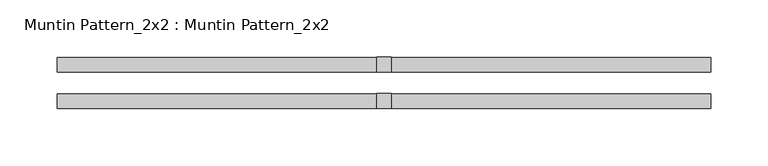
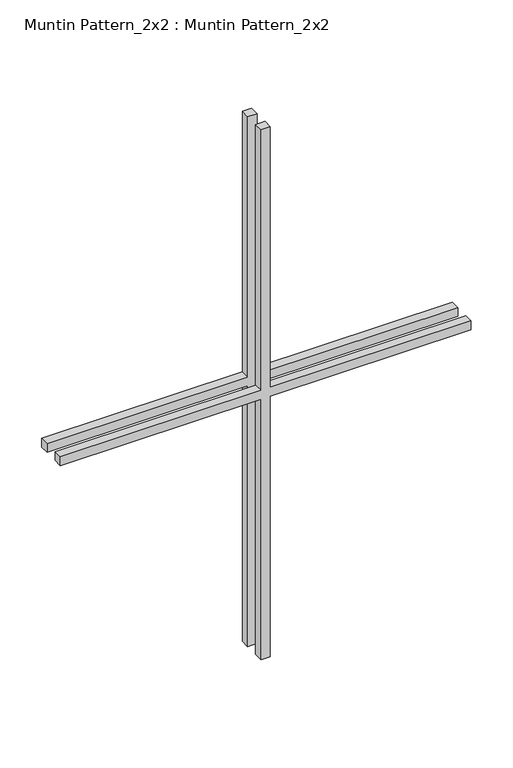
"""IFC4 building model written with IfcOpenShell, lengths in millimetres: proxy geometry, Muntin Pattern_2x2 : Muntin Pattern_2x2."""

from ifc_helpers import new_model, si_unit, frame, origin, place, context, project, spatial, polyline, outline, extrude, source, transform, mapped, element, save


def muntin_pattern_2x2_muntin_pattern_2x2_a154cbfa(model_context):
    return source(origin(), model_context, "Body", "SweptSolid", [
        extrude(outline(polyline([(393.7, -6.35), (393.7, -284.1625), (381.0, -284.1625), (381.0, -6.35), (0.0, -6.35), (0.0, 6.35), (381.0, 6.35), (381.0, 284.1625), (393.7, 284.1625), (393.7, 6.35), (774.7, 6.35), (774.7, -6.35), (393.7, -6.35)])), frame((0.0, 9.525, 0.0), z_axis=(0.0, 1.0, 0.0), x_axis=(0.0, 0.0, 1.0)), (0.0, 0.0, 1.0), 12.7),
        extrude(outline(polyline([(393.7, -6.35), (393.7, -284.1625), (381.0, -284.1625), (381.0, -6.35), (0.0, -6.35), (0.0, 6.35), (381.0, 6.35), (381.0, 284.1625), (393.7, 284.1625), (393.7, 6.35), (774.7, 6.35), (774.7, -6.35), (393.7, -6.35)])), frame((0.0, -22.225, 0.0), z_axis=(0.0, 1.0, 0.0), x_axis=(0.0, 0.0, 1.0)), (0.0, 0.0, 1.0), 12.7),
    ])


if __name__ == "__main__":
    model = new_model("IFC4")
    model_context = context("Model", 3, world=origin())
    ifc_project = project(units=[si_unit("LENGTHUNIT", "METRE", prefix="MILLI")], contexts=[model_context])
    site = spatial("IfcSite", under=ifc_project)
    building = spatial("IfcBuilding", under=site)
    placement = place(None, origin())
    muntin_pattern_2x2_muntin_pattern_2x2_shape = muntin_pattern_2x2_muntin_pattern_2x2_a154cbfa(model_context)
    element("IfcBuildingElementProxy", 1, Name="Muntin Pattern_2x2 : Muntin Pattern_2x2", ObjectType="Muntin Pattern_2x2 : Muntin Pattern_2x2", at=placement, inside=building, context=model_context, shape_type="MappedRepresentation", body=[
        mapped(muntin_pattern_2x2_muntin_pattern_2x2_shape, transform((0.0, 0.0, 0.0), x_axis=(1.0, 0.0, 0.0), y_axis=(0.0, 1.0, 0.0), z_axis=(0.0, 0.0, 1.0))),
    ])
    save(model, "model.ifc")

# Revit data of these elements
# Type "Muntin Pattern_2x2 : Muntin Pattern_2x2"
#   Width [instance default] = 4' - 0"
#   Thickness = 0' - 0 1/2"
#   Height [instance default] = 4' - 0"
#   Distance = 0' - 0 3/4"
#   Interior Material [instance default] = none
#   Exterior Material [instance default] = none
#   Default Elevation = 0
# Element 1 (IfcBuildingElementProxy, "Muntin Pattern_2x2 : Muntin Pattern_2x2")
#   Width = 1' - 10 3/8"
#   Height = 2' - 6 1/2"
#   Interior Material = Wood - Stained
#   Exterior Material = Clad - White
#   Materials on its faces: "Clad - White", "Wood - Stained"
# Materials
#   "Clad - White": class "Wood", colour RGB 242 242 238, transparency 0, Cost = 0
#   "Wood - Stained": class "Wood", colour RGB 224 178 126, transparency 0, Cost = 0
